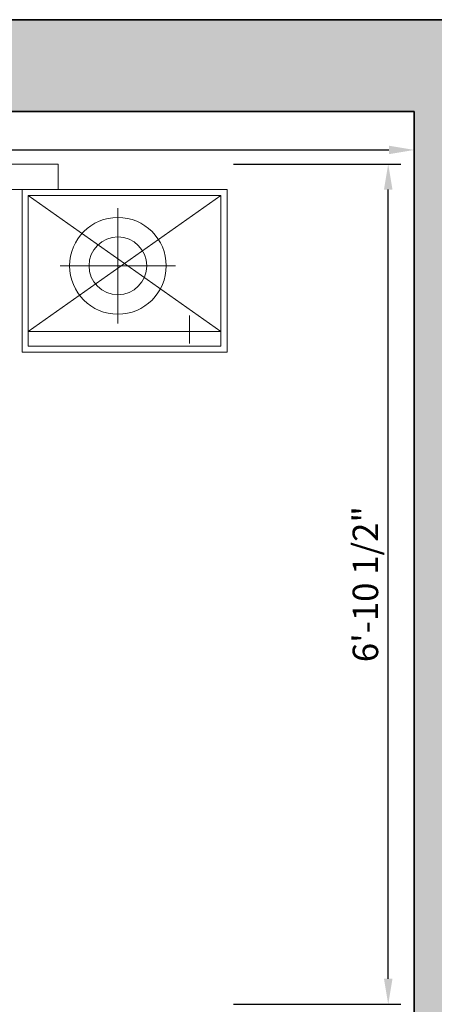
# Model space of a CAD drawing. Units: inches. Extents: x 2901 to 5923, y 918 to 2827.
# Tile 7 of 16: x 4544 to 4585, y 1534 to 1630. Entities that reach past the tile are written whole.
import ezdxf

# ---------------------------------------------------------------- set-up
doc = ezdxf.new("R2010")
doc.units = ezdxf.units.IN
for name, color, linetype, lineweight in [('A-ANNO-DIMS', 2, 'Continuous', 18), ('A-WALL-PATT', 7, 'Continuous', 13), ('furniture', 160, 'Continuous', 18), ('walls', 7, 'Continuous', 35)]:
    doc.layers.add(name, color=color, linetype=linetype, lineweight=lineweight)
doc.styles.get("Standard").update_dxf_attribs({"font": 'arial.ttf'})
doc.dimstyles.new('Copy of ISO-25', dxfattribs={"dimtxt": 2.5, "dimasz": 2.5, "dimexe": 1.25, "dimexo": 0.625, "dimtad": 1, "dimdec": 1, "dimlunit": 4, "dimtxsty": 'Standard', "dimcen": 2.5, "dimadec": 0, "dimazin": 0, "dimtfac": 1, "dimtdec": 1, "dimtmove": 0, "dimatfit": 3, "dimfxl": 1, "dimarcsym": 0})

# ---------------------------------------------------------------- blocks, each defined once
blk = doc.blocks.new('A$C029D5C69')
for p, q in [((2.2315, 2.0693), (0.4164, 2.0693)), ((2.2315, 2.0066), (2.2315, 2.0693)), ((0.4164, 2.0066), (2.2315, 2.0066)), ((2.6479, 2.0066), (2.1429, 2.0066)), ((2.1429, 2.0066), (2.1429, 1.606)), ((2.6328, 1.9915), (2.158, 1.9915)), ((2.158, 1.9915), (2.158, 1.6211)), ((2.6328, 1.6211), (2.6328, 1.9915)), ((2.6479, 1.606), (2.6479, 2.0066)), ((2.379, 1.9609), (2.379, 1.6764)), ((2.2367, 1.8186), (2.5212, 1.8186)), ((2.5551, 1.6275), (2.5551, 1.696)), ((2.1429, 1.606), (2.6479, 1.606)), ((2.158, 1.6211), (2.6328, 1.6211))]:
    blk.add_line(p, q)
at = {"ltscale": 0.005}
for p, q in [((2.6328, 1.6568), (2.158, 1.9915)), ((2.158, 1.6568), (2.6328, 1.9915)), ((2.6328, 1.6568), (2.158, 1.6568))]:
    blk.add_line(p, q, dxfattribs=at)
for radius in [0.1191, 0.0711]:
    blk.add_circle((2.379, 1.8186), radius)
blk = doc.blocks.new('A$C0D3A6DFA')
blk.add_blockref('A$C029D5C69', (0, 0))
blk = doc.blocks.new('*D36')
at = {"layer": 'A-ANNO-DIMS', "color": 0, "lineweight": -2, "transparency": 16777216}
for p, q in [((4430.068, 1631.022), (4430.068, 1640.2)), ((4892.068, 1631.022), (4892.068, 1640.2)), ((4432.568, 1638.95), (4889.568, 1638.95))]:
    blk.add_line(p, q, dxfattribs=at)
at = {"layer": 'A-ANNO-DIMS', "color": 0, "transparency": 16777216}
for points in [[(4432.568, 1639.367), (4432.568, 1638.533), (4430.068, 1638.95)], [(4889.568, 1639.367), (4889.568, 1638.533), (4892.068, 1638.95)]]:
    blk.add_solid(points, dxfattribs=at)
at = {"layer": 'Defpoints', "color": 0, "transparency": 16777216}
for p in [(4892.068, 1638.95), (4430.068, 1630.397), (4892.068, 1630.397)]:
    blk.add_point(p, dxfattribs=at)
at = {"layer": 'A-ANNO-DIMS', "color": 0, "transparency": 16777216, "insert": (4661.068, 1640.852), "char_height": 2.5, "attachment_point": 5}
blk.add_mtext('38\'-6"', dxfattribs=at)
blk = doc.blocks.new('*D39')
at = {"layer": 'A-ANNO-DIMS', "color": 0, "lineweight": -2, "transparency": 16777216}
for p, q in [((4439.068, 1620.772), (4439.068, 1616.368)), ((4583.068, 1620.772), (4583.068, 1616.368)), ((4441.568, 1617.618), (4580.568, 1617.618))]:
    blk.add_line(p, q, dxfattribs=at)
at = {"layer": 'A-ANNO-DIMS', "color": 0, "transparency": 16777216}
for points in [[(4441.568, 1618.034), (4441.568, 1617.201), (4439.068, 1617.618)], [(4580.568, 1618.034), (4580.568, 1617.201), (4583.068, 1617.618)]]:
    blk.add_solid(points, dxfattribs=at)
at = {"layer": 'Defpoints', "color": 0, "transparency": 16777216}
for p in [(4439.068, 1621.397), (4583.068, 1621.397), (4583.068, 1617.618)]:
    blk.add_point(p, dxfattribs=at)
at = {"layer": 'A-ANNO-DIMS', "color": 0, "transparency": 16777216, "insert": (4511.068, 1619.498), "char_height": 2.5, "attachment_point": 5}
blk.add_mtext("12'", dxfattribs=at)
blk = doc.blocks.new('*D82')
at = {"layer": 'A-ANNO-DIMS', "color": 0, "lineweight": -2, "transparency": 16777216}
for p, q in [((4565.309, 1616.236), (4581.757, 1616.236)), ((4580.507, 1536.296), (4580.507, 1613.736)), ((4565.309, 1533.796), (4581.757, 1533.796))]:
    blk.add_line(p, q, dxfattribs=at)
at = {"layer": 'A-ANNO-DIMS', "color": 0, "transparency": 16777216}
for points in [[(4580.091, 1613.736), (4580.924, 1613.736), (4580.507, 1616.236)], [(4580.091, 1536.296), (4580.924, 1536.296), (4580.507, 1533.796)]]:
    blk.add_solid(points, dxfattribs=at)
at = {"layer": 'Defpoints', "color": 0, "transparency": 16777216}
for p in [(4564.684, 1616.236), (4580.507, 1616.236), (4564.684, 1533.796)]:
    blk.add_point(p, dxfattribs=at)
at = {"layer": 'A-ANNO-DIMS', "color": 0, "transparency": 16777216, "insert": (4578.59, 1575.016), "char_height": 2.5, "attachment_point": 5, "rotation": 90}
blk.add_mtext('6\'-10 1/2"', dxfattribs=at)

msp = doc.modelspace()

# ---------------------------------------------------------------- hatches: boundary and pattern name
at = {"layer": 'A-WALL-PATT'}
h = msp.add_hatch(color=256, dxfattribs=at)
h.dxf.hatch_style = 1
h.paths.add_polyline_path([(4439.068, 1447.397), (4583.068, 1447.397), (4583.068, 1340.397), (4589.068, 1340.397), (4589.068, 1453.397), (4589.068, 1455.386), (4583.068, 1455.386), (4583.068, 1453.397), (4439.068, 1453.397), (4439.068, 1501.839), (4430.068, 1501.839), (4430.068, 1399.397), (4439.068, 1399.397)])
h.paths.add_polyline_path([(4439.068, 1621.397), (4487.068, 1621.397), (4487.068, 1630.397), (4430.068, 1630.397), (4430.068, 1561.839), (4439.068, 1561.839)])
h.paths.add_polyline_path([(4630.605, 1630.397), (4535.068, 1630.397), (4535.068, 1621.397), (4583.068, 1621.397), (4583.068, 1495.397), (4589.068, 1495.397), (4637.068, 1495.397), (4637.068, 1501.397), (4589.068, 1501.397), (4589.068, 1621.397), (4630.605, 1621.397)])
h.paths.add_polyline_path([(4892.068, 1630.397), (4690.605, 1630.397), (4690.605, 1621.397), (4733.068, 1621.397), (4733.068, 1564.397), (4739.068, 1564.397), (4739.068, 1621.397), (4883.068, 1621.397), (4883.068, 1528.397), (4739.068, 1528.397), (4733.068, 1528.397), (4733.068, 1501.397), (4685.068, 1501.397), (4685.068, 1495.397), (4739.068, 1495.397), (4739.068, 1519.397), (4787.068, 1519.397), (4787.068, 1423.397), (4739.068, 1423.397), (4739.068, 1456.668), (4733.068, 1456.668), (4733.068, 1340.397), (4739.068, 1340.397), (4739.068, 1417.397), (4787.068, 1417.397), (4793.068, 1417.397), (4793.068, 1423.397), (4793.068, 1519.397), (4883.068, 1519.397), (4883.068, 1482.87), (4892.068, 1482.87)])
h.paths.add_polyline_path([(4892.068, 1458.87), (4883.068, 1458.87), (4883.068, 1423.397), (4823.068, 1423.397), (4823.068, 1417.397), (4883.068, 1417.397), (4883.068, 1363.306), (4892.068, 1363.306)], flags=17)
h.paths.add_polyline_path([(4892.068, 1303.306), (4883.068, 1303.306), (4883.068, 1255.397), (4739.068, 1255.397), (4739.068, 1304.397), (4733.068, 1304.397), (4733.068, 1303.397), (4733.068, 1297.397), (4733.068, 1255.397), (4733.068, 1248.397), (4811.068, 1248.397), (4811.068, 1212.161), (4820.068, 1212.161), (4820.068, 1248.397), (4892.068, 1248.397)])
h.paths.add_polyline_path([(4820.068, 1182.161), (4811.068, 1182.161), (4811.068, 1152.397), (4685.068, 1152.397), (4685.068, 1147.029), (4685.068, 1143.397), (4733.068, 1143.397), (4811.068, 1143.397), (4814.068, 1143.397), (4820.068, 1143.397)])
h.paths.add_polyline_path([(4637.068, 1152.397), (4589.068, 1152.397), (4589.068, 1153.397), (4583.863, 1153.397), (4583.068, 1153.397), (4583.068, 1152.397), (4511.068, 1152.397), (4511.068, 1182.161), (4502.068, 1182.161), (4502.068, 1143.397), (4568.068, 1143.397), (4583.068, 1143.397), (4583.068, 1023.397), (4739.068, 1023.397), (4739.068, 1143.397), (4733.068, 1143.397), (4733.068, 1029.397), (4589.068, 1029.397), (4589.068, 1143.397), (4637.068, 1143.397), (4637.068, 1146.969)])
h.paths.add_polyline_path([(4511.068, 1246.397), (4583.068, 1246.397), (4583.068, 1188.397), (4589.068, 1188.397), (4589.068, 1246.397), (4589.068, 1248.397), (4589.068, 1255.397), (4589.068, 1297.397), (4697.068, 1297.397), (4697.068, 1303.397), (4589.068, 1303.397), (4589.068, 1304.397), (4583.068, 1304.397), (4583.068, 1255.397), (4439.068, 1255.397), (4439.068, 1261.397), (4439.068, 1351.397), (4430.068, 1351.397), (4430.068, 1252.397), (4430.068, 1246.397), (4439.068, 1246.397), (4487.068, 1246.397), (4502.068, 1246.397), (4502.068, 1212.161), (4511.068, 1212.161)])

# ---------------------------------------------------------------- linework, layer by layer
at = {"layer": 'walls'}
for p, q in [((4439.068, 1621.397), (4583.068, 1621.397)), ((4583.068, 1621.397), (4535.068, 1621.397)), ((4583.068, 1621.397), (4583.068, 1495.397))]:
    msp.add_line(p, q, dxfattribs=at)
for points in [[(4892.068, 1630.397), (4430.068, 1630.397), (4430.068, 1252.397)], [(4583.068, 1621.397), (4439.068, 1621.397), (4439.068, 1453.397)]]:
    msp.add_lwpolyline(points, dxfattribs=at)

# ---------------------------------------------------------------- block references
at = {"layer": 'furniture', "xscale": 39.84014367312396, "yscale": 39.84014367312396, "zscale": 39.84014367312396}
msp.add_blockref('A$C0D3A6DFA', (4459.192, 1533.796), dxfattribs=at)

# ---------------------------------------------------------------- dimensions: what is measured, and where the dimension line sits
at = {"layer": 'A-ANNO-DIMS'}
for base, p1, p2, picture, middle in [((4892.068, 1638.95), (4430.068, 1630.397), (4892.068, 1630.397), '*D36', (4661.068, 1640.852)), ((4583.068, 1617.618), (4439.068, 1621.397), (4583.068, 1621.397), '*D39', (4511.068, 1619.498))]:
    dim = msp.add_linear_dim(base=base, p1=p1, p2=p2, dimstyle='Copy of ISO-25', override={"dimclrd": 0, "dimclre": 0, "dimclrt": 0}, dxfattribs=at)
    dim.commit()
    dim.dimension.update_dxf_attribs({"geometry": picture, "text_midpoint": middle})
dim = msp.add_linear_dim(base=(4580.507, 1616.236), p1=(4564.684, 1533.796), p2=(4564.684, 1616.236), angle=90, dimstyle='Copy of ISO-25', override={"dimdec": 1, "dimlfac": 1, "dimrnd": 0, "dimzin": 1, "dimdsep": 46, "dimlunit": 4, "dimfrac": 2}, dxfattribs=at)
dim.commit()
dim.dimension.update_dxf_attribs({"geometry": '*D82', "text_midpoint": (4578.59, 1575.016)})

doc.saveas('drawing.dxf')
